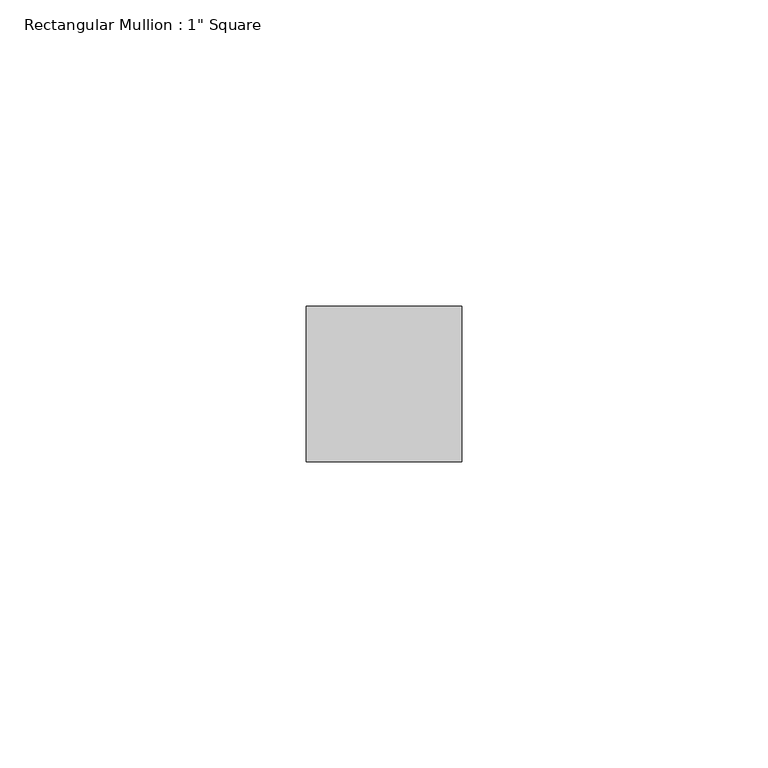
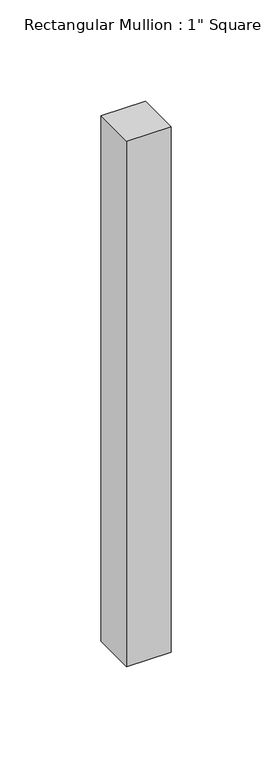
"""IFC4 building model written with IfcOpenShell, lengths in millimetres: member geometry."""

from ifc_helpers import new_model, si_unit, frame, origin, place, context, project, spatial, polyline, outline, extrude, source, transform, mapped, element, save


def member_bdd069ac(model_context):
    return source(origin(), model_context, "Body", "SweptSolid", [
        extrude(outline(polyline([(12.7, 12.7), (12.7, -12.7), (-12.7, -12.7), (-12.7, 12.7), (12.7, 12.7)])), frame((0.0, 0.0, -317.5), z_axis=(0.0, 0.0, 1.0), x_axis=(1.0, 0.0, 0.0)), (0.0, 0.0, 1.0), 317.5),
    ])


if __name__ == "__main__":
    model = new_model("IFC4")
    model_context = context("Model", 3, world=origin())
    ifc_project = project(units=[si_unit("LENGTHUNIT", "METRE", prefix="MILLI")], contexts=[model_context])
    site = spatial("IfcSite", under=ifc_project)
    building = spatial("IfcBuilding", under=site)
    placement = place(None, origin())
    member_shape = member_bdd069ac(model_context)
    element("IfcMember", 1, ObjectType="Rectangular Mullion : 1\" Square", at=placement, inside=building, context=model_context, shape_type="MappedRepresentation", body=[
        mapped(member_shape, transform((0.0, 0.0, 0.0), x_axis=(1.0, 0.0, 0.0), y_axis=(0.0, 1.0, 0.0), z_axis=(0.0, 0.0, 1.0))),
    ])
    save(model, "model.ifc")

# Revit data of these elements
# Type "Rectangular Mullion : 1\" Square"
#   built-in parameter 1007304 = 0.0833333 (stored number, unit not read)
#   built-in parameter 1007301 = 0.0416667 (stored number, unit not read)
#   built-in parameter 1007300 = 0.0416667 (stored number, unit not read)
# Element 1 (IfcMember, "Rectangular Mullion : 1\" Square")
#   Materials on its faces: "Aluminum"
# Materials
#   "Aluminum": class "Metal", colour RGB 247 247 247, transparency 0, Description = "Aluminum 6061", Cost = 0
